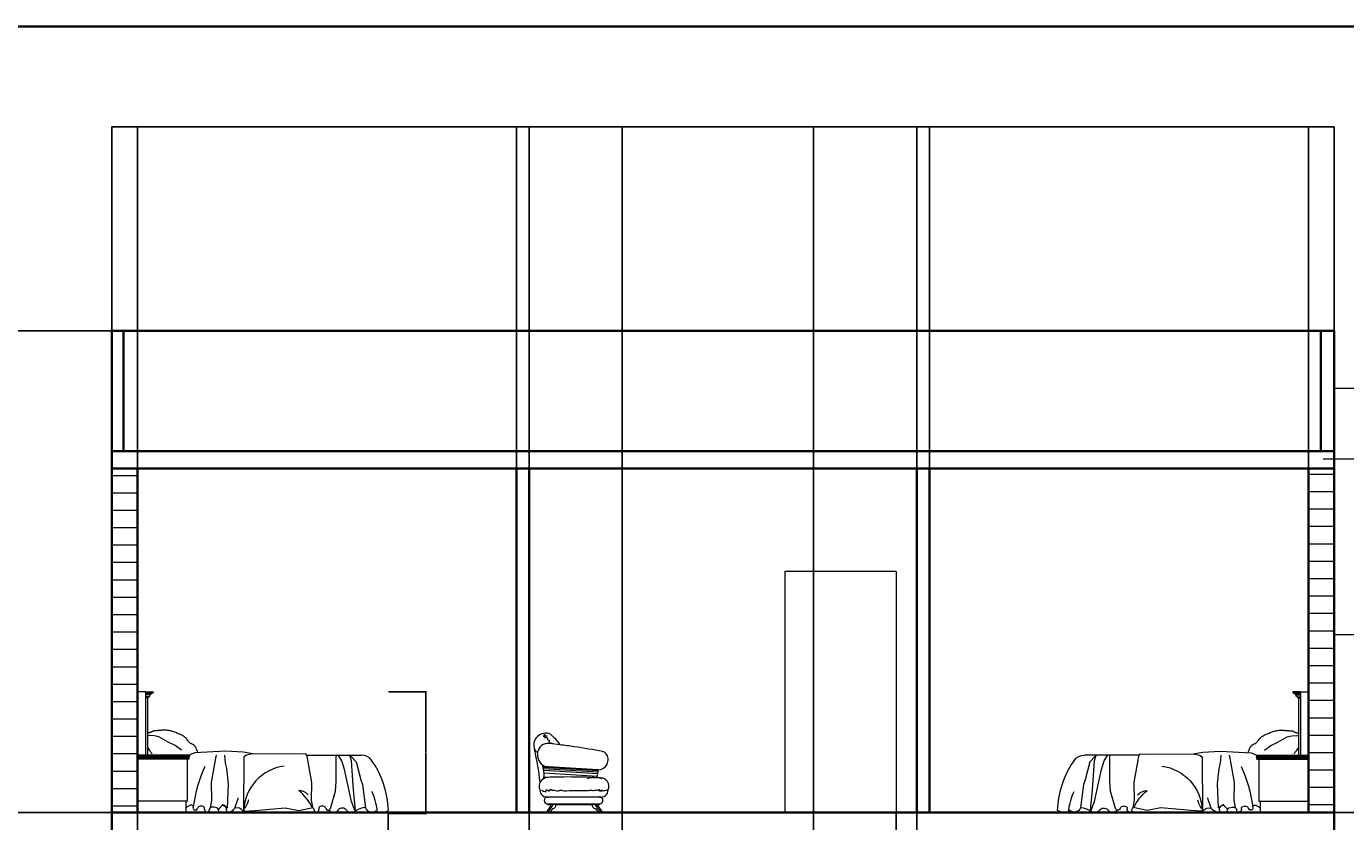
# Model space of a CAD drawing. Units: inches. Extents: x 1355 to 2746, y 1171 to 2751.
# Tile 23 of 24: x 2051 to 2510, y 2474 to 2751. Entities that reach past the tile are written whole.
import ezdxf

# ---------------------------------------------------------------- set-up
doc = ezdxf.new("R2010")
doc.units = ezdxf.units.IN
for name, color, linetype, lineweight in [('A-ANNO-DIMS', 2, 'Continuous', 18), ('A-ANNO-TEXT', 7, 'Continuous', 18), ('A-ANNO-TTLB', 7, 'Continuous', 35), ('A-FURN', 8, 'Continuous', 13), ('A-SECT', 7, 'Continuous', 35), ('A-SECT-DOOR', 3, 'Continuous', 18), ('A-WALL-PATT', 252, 'Continuous', 13)]:
    doc.layers.add(name, color=color, linetype=linetype, lineweight=lineweight)
doc.styles.get("Standard").update_dxf_attribs({"font": 'arial.ttf'})
doc.dimstyles.get("Standard").update_dxf_attribs({"dimtxt": 0.18, "dimasz": 0.18, "dimexe": 0.18, "dimexo": 0.0625, "dimgap": 0.09, "dimtad": 0, "dimtih": 1, "dimtoh": 1, "dimdec": 4, "dimzin": 0, "dimdsep": 46, "dimtxsty": 'Standard', "dimcen": 0.09, "dimadec": 0, "dimazin": 0, "dimtfac": 1, "dimtdec": 4, "dimtofl": 0, "dimtmove": 0, "dimatfit": 3, "dimfxl": 1, "dimtolj": 1, "dimtzin": 0, "dimarcsym": 0})

# ---------------------------------------------------------------- blocks, each defined once
blk = doc.blocks.new('A$C2FF713C3')
for p, q in [((0, 1050), (0, 0)), ((70, 1050), (0, 1050)), ((70, 1050), (70, 500)), ((70, 1050), (134, 1050)), ((127, 1044), (70, 1044)), ((126, 1038), (70, 1038)), ((127, 1038), (126, 1038)), ((134, 1044), (127, 1044)), ((127, 1044), (127, 1038)), ((134, 1050), (134, 1044)), ((109, 1024), (70, 1024)), ((91, 1007), (70, 1007)), ((91, 1000), (70, 1000)), ((85, 1000), (85, 500)), ((98, 1007), (91, 1007)), ((91, 1007), (91, 1000)), ((87, 693), (84, 693)), ((91, 694), (87, 693)), ((95, 694), (91, 694)), ((99, 695), (95, 694)), ((103, 696), (99, 695)), ((107, 697), (103, 696)), ((111, 698), (107, 697)), ((115, 700), (111, 698)), ((118, 701), (115, 700)), ((122, 703), (118, 701)), ((125, 704), (122, 703)), ((129, 706), (125, 704)), ((132, 708), (129, 706)), ((135, 709), (132, 708)), ((138, 710), (135, 709)), ((141, 711), (138, 710)), ((143, 712), (141, 711)), ((146, 712), (143, 712)), ((148, 712), (146, 712)), ((151, 713), (148, 712)), ((154, 713), (151, 713)), ((157, 713), (154, 713)), ((161, 713), (157, 713)), ((165, 713), (161, 713)), ((170, 713), (165, 713)), ((176, 714), (170, 713)), ((182, 714), (176, 714)), ((189, 715), (182, 714)), ((196, 716), (189, 715)), ((204, 716), (196, 716)), ((212, 717), (204, 716)), ((220, 717), (212, 717)), ((229, 717), (220, 717)), ((237, 717), (229, 717)), ((246, 717), (237, 717)), ((254, 717), (246, 717)), ((263, 716), (254, 717)), ((272, 715), (263, 716)), ((281, 713), (272, 715)), ((289, 711), (281, 713)), ((298, 709), (289, 711)), ((307, 706), (298, 709)), ((315, 703), (307, 706)), ((324, 700), (315, 703)), ((332, 697), (324, 700)), ((341, 693), (332, 697)), ((349, 690), (341, 693)), ((357, 687), (349, 690)), ((107, 672), (85, 669)), ((144, 668), (107, 672)), ((184, 660), (144, 668)), ((267, 615), (184, 660)), ((328, 585), (267, 615)), ((381, 545), (328, 585)), ((364, 684), (357, 687)), ((372, 680), (364, 684)), ((379, 677), (372, 680)), ((386, 674), (379, 677)), ((393, 670), (386, 674)), ((400, 667), (393, 670)), ((406, 662), (400, 667)), ((412, 657), (406, 662)), ((418, 651), (412, 657)), ((424, 645), (418, 651)), ((429, 639), (424, 645)), ((434, 632), (429, 639)), ((439, 626), (434, 632)), ((444, 620), (439, 626)), ((448, 614), (444, 620)), ((452, 610), (448, 614)), ((456, 606), (452, 610)), ((460, 603), (456, 606)), ((464, 601), (460, 603)), ((468, 599), (464, 601)), ((472, 598), (468, 599)), ((476, 596), (472, 598)), ((480, 594), (476, 596)), ((484, 592), (480, 594)), ((488, 590), (484, 592)), ((493, 586), (488, 590)), ((497, 581), (493, 586)), ((502, 574), (497, 581)), ((508, 565), (502, 574)), ((450, 500), (0, 500)), ((450, 488), (0, 488)), ((449, 477), (0, 477)), ((447, 465), (0, 465)), ((85, 568), (94, 556)), ((94, 556), (101, 546)), ((101, 546), (106, 539)), ((106, 539), (110, 533)), ((110, 533), (114, 528)), ((114, 528), (118, 523)), ((118, 523), (122, 518)), ((122, 518), (127, 511)), ((432, 465), (432, 100)), ((496, 522), (450, 500)), ((767, 534), (496, 522)), ((513, 553), (508, 565)), ((519, 539), (513, 553)), ((526, 521), (519, 539)), ((643, 263), (679, 473)), ((679, 473), (687, 500)), ((764, 432), (758, 500)), ((919, 526), (767, 534)), ((1001, 512), (919, 526)), ((923, 485), (920, 14)), ((948, 500), (923, 485)), ((1001, 512), (948, 500)), ((1422, 508), (1001, 512)), ((1463, 512), (1422, 508)), ((1471, 500), (1463, 512)), ((1479, 473), (1471, 500)), ((1471, 500), (1951, 500)), ((1516, 263), (1479, 473)), ((1726, 370), (1726, 500)), ((1777, 451), (1743, 502)), ((1861, 451), (1846, 500)), ((1854, 491), (1902, 443)), ((775, 385), (764, 432)), ((790, 252), (775, 385)), ((1726, 271), (1726, 370)), ((1799, 377), (1777, 451)), ((1861, 98), (1799, 377)), ((1876, 238), (1861, 451)), ((1902, 443), (1942, 285)), ((646, 109), (643, 263)), ((786, 109), (790, 252)), ((1512, 109), (1516, 263)), ((1722, 186), (1726, 271)), ((1883, 135), (1876, 238)), ((1942, 285), (1957, 245)), ((1957, 245), (1981, 42)), ((845, 40), (874, 124)), ((874, 124), (875, 130)), ((1677, 36), (1722, 186)), ((1891, 57), (1883, 135)), ((432, 100), (0, 100)), ((0, 0), (420, 0)), ((420, 100), (420, 0)), ((634, 44), (646, 109)), ((735, 72), (782, 43)), ((782, 43), (786, 109)), ((920, 14), (1022, 19)), ((956, 83), (932, 37)), ((964, 113), (956, 83)), ((1022, 19), (1283, 42)), ((1283, 42), (1402, 18)), ((1402, 18), (1524, 44)), ((1524, 44), (1512, 109)), ((1892, 12), (1861, 98)), ((1895, 14), (1891, 57))]:
    blk.add_line(p, q)
for centre, radius, start, end in [((125, 1021), 16.8, 87.4212, 169.929), ((90, 1024), 18.5, 293.7928, 1.5008), ((436, 473), 13.6, 324.9774, 17.9545), ((443, 484), 8.28, 310.9941, 35.0512), ((447, 494), 6.6, 294.6112, 65.3888), ((1951, 400), 100, 35.832, 90), ((1397, 0), 784, 1.457, 35.832), ((1735, -117), 1262, 155.6902, 172.2902), ((1328, 4), 405, 97.5724, 178.0202), ((1400, 81), 112, 40.7088, 88.9264), ((1126, -139), 433, 25.5693, 50.2938), ((1449, -73), 643, 8.3744, 23.7338), ((260, 249), 262, 307.6312, 310.5669), ((478, -13), 79.2, 115.9381, 127.154), ((517, -94), 169, 111.7814, 115.9381), ((474, 14), 53.3, 104.378, 111.7814), ((466, 46), 19.5, 71.5824, 104.378), ((465, 42), 24.2, 42.229, 71.5824), ((491, 40), 10.2, 140.3102, 217.2793), ((476, 52), 9.23, 320.3102, 42.229), ((514, 57), 39, 217.2793, 233.1579), ((501, 40), 17.5, 233.1579, 256.9409), ((501, 39), 17.2, 256.9409, 270), ((501, 74), 51.8, 270, 277.5153), ((505, 39), 16, 277.5153, 349.7827), ((546, 31), 25.7, 114.2927, 169.7827), ((554, 13), 45.2, 90, 114.2927), ((554, 21), 37.9, 63.4272, 90), ((562, 36), 20.3, 346.0902, 63.4272), ((602, 27), 20.3, 166.0902, 243.5813), ((610, 43), 38.3, 243.5813, 251.5824), ((612, 51), 46.9, 251.5824, 258.8111), ((606, 21), 16.5, 258.8111, 1.7578), ((649, 22), 25.9, 104.5937, 181.7578), ((659, -16), 65.2, 63.4581, 104.5937), ((673, 13), 33.4, 4.6698, 63.4581), ((674, 84), 58.7, 296.8941, 314.4523), ((677, 13), 29, 350.6484, 4.6698), ((713, 7), 7.4, 170.6484, 198.6345), ((712, 7), 5.58, 198.6345, 218.4296), ((208, 559), 725, 314.4523, 314.9709), ((576, 191), 204, 314.9709, 315.949), ((697, 74), 35.6, 315.949, 329.8173), ((762, 36), 40.4, 136.799, 149.8173), ((741, 56), 10.9, 81.878, 136.799), ((738, 36), 30.8, 50.0773, 81.878), ((736, 33), 34.7, 33.7168, 50.0773), ((690, 3), 89.5, 23.5428, 33.7168), ((748, 28), 26.6, 343.6974, 23.5428), ((788, 16), 15.9, 163.6974, 216.058), ((784, 13), 10.2, 216.058, 282.9819), ((759, 119), 119, 282.9819, 301.5385), ((783, 80), 73.8, 301.5385, 318.3377), ((783, 80), 74.3, 318.3377, 326.7067), ((864, -27), 69.2, 36.6754, 105.7915), ((958, 57), 57.3, 227.995, 228.6577), ((1510, 22), 25.9, 358.2422, 61.1681), ((1552, 21), 16.5, 178.2422, 281.1889), ((1546, 51), 46.9, 281.1889, 288.4176), ((1549, 43), 38.3, 288.4176, 296.4187), ((1557, 27), 20.3, 296.4187, 13.9098), ((1596, 36), 20.3, 116.5728, 193.9098), ((1604, 21), 37.9, 90, 116.5728), ((1604, 13), 45.2, 65.7073, 90), ((1612, 31), 25.7, 10.2173, 65.7073), ((1653, 39), 16, 190.2173, 262.4847), ((1658, 74), 51.8, 262.4847, 270), ((1658, 39), 17.2, 270, 283.0591), ((1658, 40), 17.5, 283.0591, 306.8421), ((1705, 43), 43.5, 208.0597, 320.5306), ((1645, 57), 39, 306.8421, 322.7207), ((1668, 40), 10.2, 322.7207, 344.9141), ((1780, -6), 46.9, 46.7208, 151.7813), ((1860, 59), 57.3, 213.2377, 312.005), ((1984, -95), 140, 91.3545, 127.5096), ((2037, 65), 60.1, 201.7886, 308.3305), ((2126, 85), 84.4, 232.0778, 309.9248)]:
    blk.add_arc(centre, radius, start, end)
blk = doc.blocks.new('A$C28ED0BDC')
for p, q in [((301, 779), (177, 793)), ((738, 491), (105, 529)), ((738, 486), (106, 524)), ((738, 481), (108, 519)), ((737, 466), (111, 504)), ((736, 446), (114, 484)), ((731, 416), (118, 453)), ((169, 180), (754, 180)), ((204, 0), (137, 0)), ((152, 10), (146, 10)), ((152, 10), (189, 10)), ((159, 100), (754, 100)), ((159, 100), (159, 95)), ((159, 95), (200, 95)), ((195, 10), (189, 10)), ((195, 10), (189, 10)), ((257, 95), (200, 95)), ((257, 95), (667, 95)), ((724, 95), (667, 95)), ((724, 95), (754, 95)), ((738, 0), (805, 0)), ((747, 10), (753, 10)), ((747, 10), (753, 10)), ((790, 10), (753, 10)), ((754, 100), (754, 95)), ((790, 10), (796, 10))]:
    blk.add_line(p, q)
for centre, radius, start, end in [((135, 776), 136, 65.3492, 202.2156), ((163, 674), 120, 83.4384, 170.9894), ((-3552, -58), 3647, 6.3782, 12.4015), ((93, 779), 99.8, 213.0962, 240.6805), ((193, 669), 151, 170.9894, 243.3914), ((737, 607), 116, 270.2622, 38.3349), ((780, 642), 60, 37.3244, 79.5985), ((-328, 419), 447, 358.1751, 17.2374), ((179, 641), 120, 243.3914, 252.6769), ((459, 479), 279, 343.505, 2.3685), ((165, 301), 103, 93.095, 202.358), ((696, 85), 316, 74.3624, 105.6376), ((764, 302), 98.3, 336.2086, 89.9815), ((152, 260), 82.4, 178.8967, 282.4453), ((159, 140), 40, 90, 270), ((771, 260), 82.4, 257.5547, 1.1033), ((754, 140), 40, 270, 90), ((149, -2), 12.3, 103.3351, 170.7152), ((-64, 190), 281, 320.2072, 340.3054), ((-29, 211), 277, 313.7174, 335.3904), ((124, 87), 101, 310.3467, 337.031), ((192, -2), 12.3, 9.2848, 76.6649), ((211, 94), 46.4, 277.4333, 1.8455), ((713, 94), 46.4, 178.1545, 262.5667), ((987, 281), 342, 213.0378, 232.5678), ((831, 152), 162, 220.1596, 241.1829), ((1022, 261), 342, 209.0488, 227.2595), ((750, -2), 12.3, 103.3351, 170.7152), ((793, -2), 12.3, 9.2848, 76.6649)]:
    blk.add_arc(centre, radius, start, end)
for points, knots in [([(124, 901), (121, 898), (113, 890), (147, 895), (73, 866), (197, 893), (86, 855), (175, 866), (142, 832), (182, 838), (163, 800), (225, 796), (220, 788)], [0, 0, 0, 0, 9.765075, 22.239713, 47.817951, 93.447543, 130.976544, 169.416587, 185.180341, 209.428428, 221.888603, 276.469797, 276.469797, 276.469797, 276.469797]), ([(301, 779), (300, 780), (270, 832), (238, 855), (192, 900)], [244.920573, 244.920573, 244.920573, 244.920573, 247.928636, 395.738949, 395.738949, 395.738949, 395.738949]), ([(791, 701), (683, 721), (520, 751), (356, 772), (301, 779)], [18.761969, 18.761969, 18.761969, 18.761969, 348.756072, 515.290542, 515.290542, 515.290542, 515.290542]), ([(764, 400), (674, 404), (398, 413), (208, 407), (107, 404)], [0, 0, 0, 0, 269.198238, 571.026582, 571.026582, 571.026582, 571.026582]), ([(93, 257), (117, 244), (148, 228), (136, 281), (184, 233), (182, 277), (214, 254), (239, 259), (267, 245), (314, 263), (326, 247), (419, 255), (548, 253), (616, 256), (660, 257)], [0, 0, 0, 0, 49.407579, 64.565784, 105.844847, 118.345477, 155.269185, 167.410003, 198.361737, 241.285001, 308.128282, 447.747709, 520.592639, 652.828768, 652.828768, 652.828768, 652.828768]), ([(849, 262), (837, 257), (814, 249), (727, 241), (827, 263), (730, 243), (771, 266), (713, 252), (687, 252), (629, 253), (589, 251), (565, 249)], [0, 0, 0, 0, 49.380651, 92.855981, 126.791693, 168.915675, 179.762432, 213.696461, 251.182, 296.320949, 372.653556, 372.653556, 372.653556, 372.653556])]:
    blk.add_open_spline(points, degree=3, knots=knots)
blk = doc.blocks.new('DOOR-OPENING-SECTION')
for p, q in [((0, 84), (0, 0)), ((38.81, 84), (0, 84)), ((38.81, 84), (38.81, 0))]:
    blk.add_line(p, q)
blk = doc.blocks.new('*D89')
at = {"layer": 'A-ANNO-DIMS', "color": 0, "lineweight": -2, "transparency": 16777216}
for p, q in [((2089.39, 2477.07), (2089.39, 2463.85)), ((2176.75, 2477.07), (2176.75, 2463.85)), ((2089.57, 2464.03), (2132.25, 2464.03)), ((2176.57, 2464.03), (2133.89, 2464.03))]:
    blk.add_line(p, q, dxfattribs=at)
at = {"layer": 'A-ANNO-DIMS', "color": 0, "transparency": 16777216}
for points in [[(2089.57, 2464.06), (2089.57, 2464), (2089.39, 2464.03)], [(2176.57, 2464.06), (2176.57, 2464), (2176.75, 2464.03)]]:
    blk.add_solid(points, dxfattribs=at)
at = {"layer": 'Defpoints', "color": 0, "transparency": 16777216}
for p in [(2089.39, 2477.13), (2176.75, 2477.13), (2176.75, 2464.03)]:
    blk.add_point(p, dxfattribs=at)
at = {"layer": 'A-ANNO-DIMS', "color": 0, "transparency": 16777216, "insert": (2133.07, 2464.03), "char_height": 0.18, "attachment_point": 5}
blk.add_mtext('\\A1;BED 87 TYP.', dxfattribs=at)
blk = doc.blocks.new('*D90')
at = {"layer": 'A-ANNO-DIMS', "color": 0, "lineweight": -2, "transparency": 16777216}
for p, q in [((2176.81, 2519.47), (2190.03, 2519.47)), ((2189.85, 2519.29), (2189.85, 2498.48)), ((2189.85, 2477.31), (2189.85, 2498.12)), ((2176.81, 2477.13), (2190.03, 2477.13))]:
    blk.add_line(p, q, dxfattribs=at)
at = {"layer": 'A-ANNO-DIMS', "color": 0, "transparency": 16777216}
for points in [[(2189.82, 2519.29), (2189.88, 2519.29), (2189.85, 2519.47)], [(2189.82, 2477.31), (2189.88, 2477.31), (2189.85, 2477.13)]]:
    blk.add_solid(points, dxfattribs=at)
at = {"layer": 'Defpoints', "color": 0, "transparency": 16777216}
for p in [(2176.75, 2519.47), (2189.85, 2519.47), (2176.75, 2477.13)]:
    blk.add_point(p, dxfattribs=at)
at = {"layer": 'A-ANNO-DIMS', "color": 0, "transparency": 16777216, "insert": (2189.85, 2498.3), "char_height": 0.18, "attachment_point": 5}
blk.add_mtext('\\A1;42 TYP.', dxfattribs=at)
blk = doc.blocks.new('*D99')
at = {"layer": 'A-ANNO-DIMS', "color": 0, "lineweight": -2, "transparency": 16777216}
for p, q in [((2080.39, 2139.36), (2080.39, 2716.58)), ((2080.57, 2716.4), (2152.75, 2716.4)), ((2225.71, 2716.4), (2153.53, 2716.4)), ((2225.89, 2139.36), (2225.89, 2716.58))]:
    blk.add_line(p, q, dxfattribs=at)
at = {"layer": 'A-ANNO-DIMS', "color": 0, "transparency": 16777216}
for points in [[(2080.57, 2716.43), (2080.57, 2716.37), (2080.39, 2716.4)], [(2225.71, 2716.43), (2225.71, 2716.37), (2225.89, 2716.4)]]:
    blk.add_solid(points, dxfattribs=at)
at = {"layer": 'Defpoints', "color": 0, "transparency": 16777216}
for p in [(2225.89, 2716.4), (2080.39, 2139.3), (2225.89, 2139.3)]:
    blk.add_point(p, dxfattribs=at)
at = {"layer": 'A-ANNO-DIMS', "color": 0, "transparency": 16777216, "insert": (2153.14, 2716.4), "char_height": 0.18, "attachment_point": 5}
blk.add_mtext('\\A1;145.5', dxfattribs=at)
blk = doc.blocks.new('*D100')
at = {"layer": 'A-ANNO-DIMS', "color": 0, "lineweight": -2, "transparency": 16777216}
for p, q in [((2225.89, 2139.36), (2225.89, 2716.58)), ((2226.07, 2716.4), (2293.11, 2716.4)), ((2360.71, 2716.4), (2293.67, 2716.4)), ((2360.89, 2139.36), (2360.89, 2716.58))]:
    blk.add_line(p, q, dxfattribs=at)
at = {"layer": 'A-ANNO-DIMS', "color": 0, "transparency": 16777216}
for points in [[(2226.07, 2716.43), (2226.07, 2716.37), (2225.89, 2716.4)], [(2360.71, 2716.43), (2360.71, 2716.37), (2360.89, 2716.4)]]:
    blk.add_solid(points, dxfattribs=at)
at = {"layer": 'Defpoints', "color": 0, "transparency": 16777216}
for p in [(2360.89, 2716.4), (2225.89, 2139.3), (2360.89, 2139.3)]:
    blk.add_point(p, dxfattribs=at)
at = {"layer": 'A-ANNO-DIMS', "color": 0, "transparency": 16777216, "insert": (2293.39, 2716.4), "char_height": 0.18, "attachment_point": 5}
blk.add_mtext('\\A1;135', dxfattribs=at)
blk = doc.blocks.new('*D101')
at = {"layer": 'A-ANNO-DIMS', "color": 0, "lineweight": -2, "transparency": 16777216}
for p, q in [((2360.89, 2139.36), (2360.89, 2716.58)), ((2361.07, 2716.4), (2433.25, 2716.4)), ((2506.21, 2716.4), (2434.03, 2716.4)), ((2506.39, 2139.36), (2506.39, 2716.58))]:
    blk.add_line(p, q, dxfattribs=at)
at = {"layer": 'A-ANNO-DIMS', "color": 0, "transparency": 16777216}
for points in [[(2361.07, 2716.43), (2361.07, 2716.37), (2360.89, 2716.4)], [(2506.21, 2716.43), (2506.21, 2716.37), (2506.39, 2716.4)]]:
    blk.add_solid(points, dxfattribs=at)
at = {"layer": 'Defpoints', "color": 0, "transparency": 16777216}
for p in [(2506.39, 2716.4), (2360.89, 2139.3), (2506.39, 2139.3)]:
    blk.add_point(p, dxfattribs=at)
at = {"layer": 'A-ANNO-DIMS', "color": 0, "transparency": 16777216, "insert": (2433.64, 2716.4), "char_height": 0.18, "attachment_point": 5}
blk.add_mtext('\\A1;145.5', dxfattribs=at)
blk = doc.blocks.new('*D112')
at = {"layer": 'A-ANNO-DIMS', "color": 0, "lineweight": -2, "transparency": 16777216}
for p, q in [((2258.27, 2095.29), (2258.27, 2716.58)), ((2258.45, 2716.4), (2291.19, 2716.4)), ((2324.72, 2716.4), (2291.98, 2716.4)), ((2324.9, 2095.29), (2324.9, 2716.58))]:
    blk.add_line(p, q, dxfattribs=at)
at = {"layer": 'A-ANNO-DIMS', "color": 0, "transparency": 16777216}
for points in [[(2258.45, 2716.43), (2258.45, 2716.37), (2258.27, 2716.4)], [(2324.72, 2716.43), (2324.72, 2716.37), (2324.9, 2716.4)]]:
    blk.add_solid(points, dxfattribs=at)
at = {"layer": 'Defpoints', "color": 0, "transparency": 16777216}
for p in [(2324.9, 2716.4), (2258.27, 2095.22), (2324.9, 2095.22)]:
    blk.add_point(p, dxfattribs=at)
at = {"layer": 'A-ANNO-DIMS', "color": 0, "transparency": 16777216, "insert": (2291.58, 2716.4), "char_height": 0.18, "attachment_point": 5}
blk.add_mtext('\\A1;66.63', dxfattribs=at)
blk = doc.blocks.new('*D116')
at = {"layer": 'A-ANNO-DIMS', "color": 0, "lineweight": -2, "transparency": 16777216}
for p, q in [((1976.77, 2477.4), (2648.07, 2477.4)), ((2647.89, 2477.22), (2647.89, 2414.58)), ((2647.89, 2351.58), (2647.89, 2414.22)), ((1976.77, 2351.4), (2648.07, 2351.4))]:
    blk.add_line(p, q, dxfattribs=at)
at = {"layer": 'A-ANNO-DIMS', "color": 0, "transparency": 16777216}
for points in [[(2647.86, 2477.22), (2647.92, 2477.22), (2647.89, 2477.4)], [(2647.86, 2351.58), (2647.92, 2351.58), (2647.89, 2351.4)]]:
    blk.add_solid(points, dxfattribs=at)
at = {"layer": 'Defpoints', "color": 0, "transparency": 16777216}
for p in [(1976.71, 2477.4), (2647.89, 2477.4), (1976.71, 2351.4)]:
    blk.add_point(p, dxfattribs=at)
at = {"layer": 'A-ANNO-DIMS', "color": 0, "transparency": 16777216, "insert": (2647.89, 2414.4), "char_height": 0.18, "attachment_point": 5}
blk.add_mtext('\\A1;126', dxfattribs=at)
blk = doc.blocks.new('*D127')
at = {"layer": 'A-ANNO-DIMS', "color": 0, "lineweight": -2, "transparency": 16777216}
for p, q in [((2080.33, 2645.4), (1407.53, 2645.4)), ((1407.71, 2645.22), (1407.71, 2432.58)), ((1407.71, 2219.58), (1407.71, 2432.22)), ((2080.33, 2219.4), (1407.53, 2219.4))]:
    blk.add_line(p, q, dxfattribs=at)
at = {"layer": 'A-ANNO-DIMS', "color": 0, "transparency": 16777216}
for points in [[(1407.68, 2645.22), (1407.74, 2645.22), (1407.71, 2645.4)], [(1407.68, 2219.58), (1407.74, 2219.58), (1407.71, 2219.4)]]:
    blk.add_solid(points, dxfattribs=at)
at = {"layer": 'Defpoints', "color": 0, "transparency": 16777216}
for p in [(1407.71, 2645.4), (2080.39, 2645.4), (2080.39, 2219.4)]:
    blk.add_point(p, dxfattribs=at)
at = {"layer": 'A-ANNO-DIMS', "color": 0, "transparency": 16777216, "insert": (1407.71, 2432.4), "char_height": 0.18, "attachment_point": 5}
blk.add_mtext('\\A1;426', dxfattribs=at)
blk = doc.blocks.new('*D128')
at = {"layer": 'A-ANNO-DIMS', "color": 0, "lineweight": -2, "transparency": 16777216}
for p, q in [((2506.45, 2477.4), (2648.07, 2477.4)), ((2647.89, 2477.22), (2647.89, 2414.58)), ((2647.89, 2351.58), (2647.89, 2414.22)), ((2506.45, 2351.4), (2648.07, 2351.4))]:
    blk.add_line(p, q, dxfattribs=at)
at = {"layer": 'A-ANNO-DIMS', "color": 0, "transparency": 16777216}
for points in [[(2647.86, 2477.22), (2647.92, 2477.22), (2647.89, 2477.4)], [(2647.86, 2351.58), (2647.92, 2351.58), (2647.89, 2351.4)]]:
    blk.add_solid(points, dxfattribs=at)
at = {"layer": 'Defpoints', "color": 0, "transparency": 16777216}
for p in [(2506.39, 2477.4), (2647.89, 2477.4), (2506.39, 2351.4)]:
    blk.add_point(p, dxfattribs=at)
at = {"layer": 'A-ANNO-DIMS', "color": 0, "transparency": 16777216, "insert": (2647.89, 2414.4), "char_height": 0.18, "attachment_point": 5}
blk.add_mtext('\\A1;126', dxfattribs=at)
blk = doc.blocks.new('*D129')
at = {"layer": 'A-ANNO-DIMS', "color": 0, "lineweight": -2, "transparency": 16777216}
for p, q in [((2089.39, 2597.46), (2089.39, 2716.58)), ((2089.57, 2716.4), (2155.11, 2716.4)), ((2221.21, 2716.4), (2155.67, 2716.4)), ((2221.39, 2597.46), (2221.39, 2716.58))]:
    blk.add_line(p, q, dxfattribs=at)
at = {"layer": 'A-ANNO-DIMS', "color": 0, "transparency": 16777216}
for points in [[(2089.57, 2716.43), (2089.57, 2716.37), (2089.39, 2716.4)], [(2221.21, 2716.43), (2221.21, 2716.37), (2221.39, 2716.4)]]:
    blk.add_solid(points, dxfattribs=at)
at = {"layer": 'Defpoints', "color": 0, "transparency": 16777216}
for p in [(2221.39, 2716.4), (2089.39, 2597.4), (2221.39, 2597.4)]:
    blk.add_point(p, dxfattribs=at)
at = {"layer": 'A-ANNO-DIMS', "color": 0, "transparency": 16777216, "insert": (2155.39, 2716.4), "char_height": 0.18, "attachment_point": 5}
blk.add_mtext('\\A1;132', dxfattribs=at)
blk = doc.blocks.new('*D130')
at = {"layer": 'A-ANNO-DIMS', "color": 0, "lineweight": -2, "transparency": 16777216}
for p, q in [((2225.89, 2597.46), (2225.89, 2716.58)), ((2226.07, 2716.4), (2293.11, 2716.4)), ((2360.71, 2716.4), (2293.67, 2716.4)), ((2360.89, 2597.46), (2360.89, 2716.58))]:
    blk.add_line(p, q, dxfattribs=at)
at = {"layer": 'A-ANNO-DIMS', "color": 0, "transparency": 16777216}
for points in [[(2226.07, 2716.43), (2226.07, 2716.37), (2225.89, 2716.4)], [(2360.71, 2716.43), (2360.71, 2716.37), (2360.89, 2716.4)]]:
    blk.add_solid(points, dxfattribs=at)
at = {"layer": 'Defpoints', "color": 0, "transparency": 16777216}
for p in [(2360.89, 2716.4), (2225.89, 2597.4), (2360.89, 2597.4)]:
    blk.add_point(p, dxfattribs=at)
at = {"layer": 'A-ANNO-DIMS', "color": 0, "transparency": 16777216, "insert": (2293.39, 2716.4), "char_height": 0.18, "attachment_point": 5}
blk.add_mtext('\\A1;135', dxfattribs=at)
blk = doc.blocks.new('*D131')
at = {"layer": 'A-ANNO-DIMS', "color": 0, "lineweight": -2, "transparency": 16777216}
for p, q in [((2365.39, 2597.46), (2365.39, 2716.58)), ((2365.57, 2716.4), (2431.11, 2716.4)), ((2497.21, 2716.4), (2431.67, 2716.4)), ((2497.39, 2597.46), (2497.39, 2716.58))]:
    blk.add_line(p, q, dxfattribs=at)
at = {"layer": 'A-ANNO-DIMS', "color": 0, "transparency": 16777216}
for points in [[(2365.57, 2716.43), (2365.57, 2716.37), (2365.39, 2716.4)], [(2497.21, 2716.43), (2497.21, 2716.37), (2497.39, 2716.4)]]:
    blk.add_solid(points, dxfattribs=at)
at = {"layer": 'Defpoints', "color": 0, "transparency": 16777216}
for p in [(2497.39, 2716.4), (2365.39, 2597.4), (2497.39, 2597.4)]:
    blk.add_point(p, dxfattribs=at)
at = {"layer": 'A-ANNO-DIMS', "color": 0, "transparency": 16777216, "insert": (2431.39, 2716.4), "char_height": 0.18, "attachment_point": 5}
blk.add_mtext('\\A1;132', dxfattribs=at)
blk = doc.blocks.new('*D132')
at = {"layer": 'A-ANNO-DIMS', "color": 0, "lineweight": -2, "transparency": 16777216}
for p, q in [((2221.39, 2597.46), (2221.39, 2716.58)), ((2221.57, 2716.4), (2223.38, 2716.4)), ((2225.71, 2716.4), (2223.9, 2716.4)), ((2225.89, 2597.46), (2225.89, 2716.58))]:
    blk.add_line(p, q, dxfattribs=at)
at = {"layer": 'A-ANNO-DIMS', "color": 0, "transparency": 16777216}
for points in [[(2221.57, 2716.43), (2221.57, 2716.37), (2221.39, 2716.4)], [(2225.71, 2716.43), (2225.71, 2716.37), (2225.89, 2716.4)]]:
    blk.add_solid(points, dxfattribs=at)
at = {"layer": 'Defpoints', "color": 0, "transparency": 16777216}
for p in [(2225.89, 2716.4), (2221.39, 2597.4), (2225.89, 2597.4)]:
    blk.add_point(p, dxfattribs=at)
at = {"layer": 'A-ANNO-DIMS', "color": 0, "transparency": 16777216, "insert": (2223.64, 2716.4), "char_height": 0.18, "attachment_point": 5}
blk.add_mtext('\\A1;4.5', dxfattribs=at)
blk = doc.blocks.new('*D133')
at = {"layer": 'A-ANNO-DIMS', "color": 0, "lineweight": -2, "transparency": 16777216}
for p, q in [((2080.39, 2597.46), (2080.39, 2716.58)), ((2080.57, 2716.4), (2084.74, 2716.4)), ((2089.21, 2716.4), (2085.04, 2716.4)), ((2089.39, 2597.46), (2089.39, 2716.58))]:
    blk.add_line(p, q, dxfattribs=at)
at = {"layer": 'A-ANNO-DIMS', "color": 0, "transparency": 16777216}
for points in [[(2080.57, 2716.43), (2080.57, 2716.37), (2080.39, 2716.4)], [(2089.21, 2716.43), (2089.21, 2716.37), (2089.39, 2716.4)]]:
    blk.add_solid(points, dxfattribs=at)
at = {"layer": 'Defpoints', "color": 0, "transparency": 16777216}
for p in [(2089.39, 2716.4), (2080.39, 2597.4), (2089.39, 2597.4)]:
    blk.add_point(p, dxfattribs=at)
at = {"layer": 'A-ANNO-DIMS', "color": 0, "transparency": 16777216, "insert": (2084.89, 2716.4), "char_height": 0.18, "attachment_point": 5}
blk.add_mtext('\\A1;9', dxfattribs=at)
blk = doc.blocks.new('*D134')
at = {"layer": 'A-ANNO-DIMS', "color": 0, "lineweight": -2, "transparency": 16777216}
for p, q in [((2353.71, 2477.34), (2353.71, 1171.06)), ((2360.89, 2477.34), (2360.89, 1171.06)), ((2353.89, 1171.24), (2356.92, 1171.24)), ((2360.71, 1171.24), (2357.68, 1171.24))]:
    blk.add_line(p, q, dxfattribs=at)
at = {"layer": 'A-ANNO-DIMS', "color": 0, "transparency": 16777216}
for points in [[(2353.89, 1171.27), (2353.89, 1171.21), (2353.71, 1171.24)], [(2360.71, 1171.27), (2360.71, 1171.21), (2360.89, 1171.24)]]:
    blk.add_solid(points, dxfattribs=at)
at = {"layer": 'Defpoints', "color": 0, "transparency": 16777216}
for p in [(2353.71, 2477.4), (2360.89, 2477.4), (2360.89, 1171.24)]:
    blk.add_point(p, dxfattribs=at)
at = {"layer": 'A-ANNO-DIMS', "color": 0, "transparency": 16777216, "insert": (2357.3, 1171.24), "char_height": 0.18, "attachment_point": 5}
blk.add_mtext('\\A1;7.181', dxfattribs=at)

msp = doc.modelspace()

# ---------------------------------------------------------------- hatches: boundary and pattern name
at = {"layer": 'A-WALL-PATT'}
h = msp.add_hatch(dxfattribs=at)
h.set_pattern_fill('ANSI31', color=256, scale=1.909606, angle=-45, style=0)
h.paths.add_polyline_path([(2080.3909, 2477.3999), (2089.3909, 2477.3999), (2089.3909, 2597.3999), (2080.3909, 2597.3999)])
h = msp.add_hatch(dxfattribs=at)
h.set_pattern_fill('ANSI31', color=256, scale=1.90992, angle=-45, style=0)
h.paths.add_polyline_path([(2497.3909, 2477.3999), (2506.3909, 2477.3999), (2506.3909, 2597.3999), (2497.3909, 2597.3999)])

# ---------------------------------------------------------------- linework, layer by layer
at = {"layer": 'A-ANNO-TEXT'}
for p, q in [((2506.3909, 2625.3279), (2529.1047, 2625.3279)), ((2502.5164, 2600.7394), (2530.7325, 2600.7394)), ((2506.3909, 2539.5356), (2506.3909, 2539.5356)), ((2506.3909, 2539.5356), (2536.1371, 2539.5356))]:
    msp.add_line(p, q, dxfattribs=at)
at = {"layer": 'A-ANNO-TTLB'}
msp.add_lwpolyline([(1355.0901, 2751.4741), (2746.1804, 2751.4741), (2746.1804, 1182.883), (1355.0901, 1182.883)], close=True, dxfattribs=at)
at = {"layer": 'A-SECT'}
for p, q in [((2080.3909, 2645.3999), (2080.3909, 2471.3999)), ((2506.3909, 2645.3999), (2080.3909, 2645.3999)), ((2084.4557, 2603.3999), (2084.4557, 2645.3999)), ((2501.6809, 2603.3999), (2501.6809, 2645.3999)), ((2506.3909, 2645.3999), (2506.3909, 2471.3999)), ((2506.3909, 2603.3999), (2080.3909, 2603.3999)), ((2506.3909, 2597.3999), (2080.3909, 2597.3999)), ((2089.3909, 2597.3999), (2089.3909, 2477.3999)), ((2221.3909, 2597.3999), (2221.3909, 2477.3999)), ((2225.8909, 2597.3999), (2225.8909, 2477.3999)), ((2360.8909, 2597.3999), (2360.8909, 2477.3999)), ((2365.3909, 2597.3999), (2365.3909, 2477.3999)), ((2497.3909, 2597.3999), (2497.3909, 2477.3999)), ((2080.3909, 2519.3999), (2080.3909, 2345.3999)), ((2506.3909, 2519.3999), (2506.3909, 2345.3999)), ((2506.3909, 2477.3999), (2080.3909, 2477.3999))]:
    msp.add_line(p, q, dxfattribs=at)

# ---------------------------------------------------------------- block references
at = {"layer": 'A-FURN'}
for name, p, xscale, yscale, zscale in [('A$C2FF713C3', (2089.3909, 2477.3801), 0.0400677785412672, 0.0400677785412672, 0.0400677785412672), ('A$C2FF713C3', (2497.3909, 2477.3801), -0.0400677785412672, 0.0400677785412672, 0.0400677785412672), ('A$C28ED0BDC', (2227.4528, 2477.3942), 0.0303702499100781, 0.0303702499100781, 0.0303702499100781)]:
    msp.add_blockref(name, p, dxfattribs=dict(at, xscale=xscale, yscale=yscale, zscale=zscale))
at = {"layer": 'A-SECT-DOOR'}
msp.add_blockref('DOOR-OPENING-SECTION', (2314.902, 2477.4), dxfattribs=at)

# ---------------------------------------------------------------- dimensions: what is measured, and where the dimension line sits
at = {"layer": 'A-ANNO-DIMS'}
for base, p1, p2, override, picture, middle in [((2225.8909, 2716.3999), (2080.3909, 2139.3018), (2225.8909, 2139.3018), {"dimdec": 1, "dimlfac": 1, "dimrnd": 0, "dimzin": 0, "dimdsep": 46, "dimlunit": 2}, '*D99', (2153.1409, 2716.3999)), ((2089.3909, 2716.3999), (2080.3909, 2597.3999), (2089.3909, 2597.3999), {"dimdec": 0, "dimlfac": 1, "dimrnd": 0, "dimzin": 0, "dimdsep": 46, "dimlunit": 2}, '*D133', (2084.8909, 2716.3999)), ((2221.3909, 2716.3999), (2089.3909, 2597.3999), (2221.3909, 2597.3999), {"dimdec": 0, "dimlfac": 1, "dimrnd": 0, "dimzin": 0, "dimdsep": 46, "dimlunit": 2}, '*D129', (2155.3909, 2716.3999)), ((2225.8909, 2716.3999), (2221.3909, 2597.3999), (2225.8909, 2597.3999), {"dimdec": 1, "dimlfac": 1, "dimrnd": 0, "dimzin": 0, "dimdsep": 46, "dimlunit": 2}, '*D132', (2223.6409, 2716.3999)), ((2360.8909, 2716.3999), (2225.8909, 2139.3018), (2360.8909, 2139.3018), {"dimdec": 0, "dimlfac": 1, "dimrnd": 0, "dimzin": 0, "dimdsep": 46, "dimlunit": 2}, '*D100', (2293.3909, 2716.3999)), ((2360.8909, 2716.3999), (2225.8909, 2597.3999), (2360.8909, 2597.3999), {"dimdec": 0, "dimlfac": 1, "dimrnd": 0, "dimzin": 0, "dimdsep": 46, "dimlunit": 2}, '*D130', (2293.3909, 2716.3999)), ((2324.8959, 2716.3999), (2258.2658, 2095.2225), (2324.8959, 2095.2225), {"dimdec": 2, "dimlfac": 1, "dimrnd": 0, "dimzin": 0, "dimdsep": 46, "dimlunit": 2}, '*D112', (2291.5809, 2716.3999)), ((2506.3909, 2716.3999), (2360.8909, 2139.3018), (2506.3909, 2139.3018), {"dimdec": 1, "dimlfac": 1, "dimrnd": 0, "dimzin": 0, "dimdsep": 46, "dimlunit": 2}, '*D101', (2433.6409, 2716.3999)), ((2497.3909, 2716.3999), (2365.3909, 2597.3999), (2497.3909, 2597.3999), {"dimdec": 0, "dimlfac": 1, "dimrnd": 0, "dimzin": 0, "dimdsep": 46, "dimlunit": 2}, '*D131', (2431.3909, 2716.3999)), ((2360.8909, 1171.2388), (2353.71, 2477.3999), (2360.8909, 2477.3999), {"dimdec": 3, "dimlfac": 1, "dimrnd": 0, "dimzin": 0, "dimdsep": 46, "dimlunit": 2}, '*D134', (2357.3004, 1171.2388))]:
    dim = msp.add_linear_dim(base=base, p1=p1, p2=p2, dimstyle='Standard', override=override, dxfattribs=at)
    dim.commit()
    dim.dimension.update_dxf_attribs({"geometry": picture, "text_midpoint": middle})
for base, p1, p2, picture, middle in [((1407.7083, 2645.3999), (2080.3909, 2219.3999), (2080.3909, 2645.3999), '*D127', (1407.7083, 2432.3999)), ((2647.886, 2477.3999), (1976.7083, 2351.3999), (1976.7083, 2477.3999), '*D116', (2647.886, 2414.3999)), ((2647.886, 2477.3999), (2506.3909, 2351.3999), (2506.3909, 2477.3999), '*D128', (2647.886, 2414.3999))]:
    dim = msp.add_linear_dim(base=base, p1=p1, p2=p2, angle=90, dimstyle='Standard', override={"dimdec": 0, "dimlfac": 1, "dimrnd": 0, "dimzin": 0, "dimdsep": 46, "dimlunit": 2}, dxfattribs=at)
    dim.commit()
    dim.dimension.update_dxf_attribs({"geometry": picture, "text_midpoint": middle})
dim = msp.add_linear_dim(base=(2189.8491, 2519.4711), p1=(2176.7459, 2477.1343), p2=(2176.7459, 2519.4711), angle=90, text='<> TYP.', dimstyle='Standard', override={"dimdec": 0, "dimlfac": 1, "dimrnd": 0, "dimzin": 0, "dimdsep": 46, "dimlunit": 2}, dxfattribs=at)
dim.commit()
dim.dimension.update_dxf_attribs({"geometry": '*D90', "text_midpoint": (2189.8491, 2498.3027)})
dim = msp.add_linear_dim(base=(2176.7459, 2464.0311), p1=(2089.3909, 2477.1343), p2=(2176.7459, 2477.1343), text='BED <> TYP.', dimstyle='Standard', override={"dimdec": 0, "dimlfac": 1, "dimrnd": 0, "dimzin": 0, "dimdsep": 46, "dimlunit": 2}, dxfattribs=at)
dim.commit()
dim.dimension.update_dxf_attribs({"geometry": '*D89', "text_midpoint": (2133.0684, 2464.0311)})

doc.saveas('drawing.dxf')
